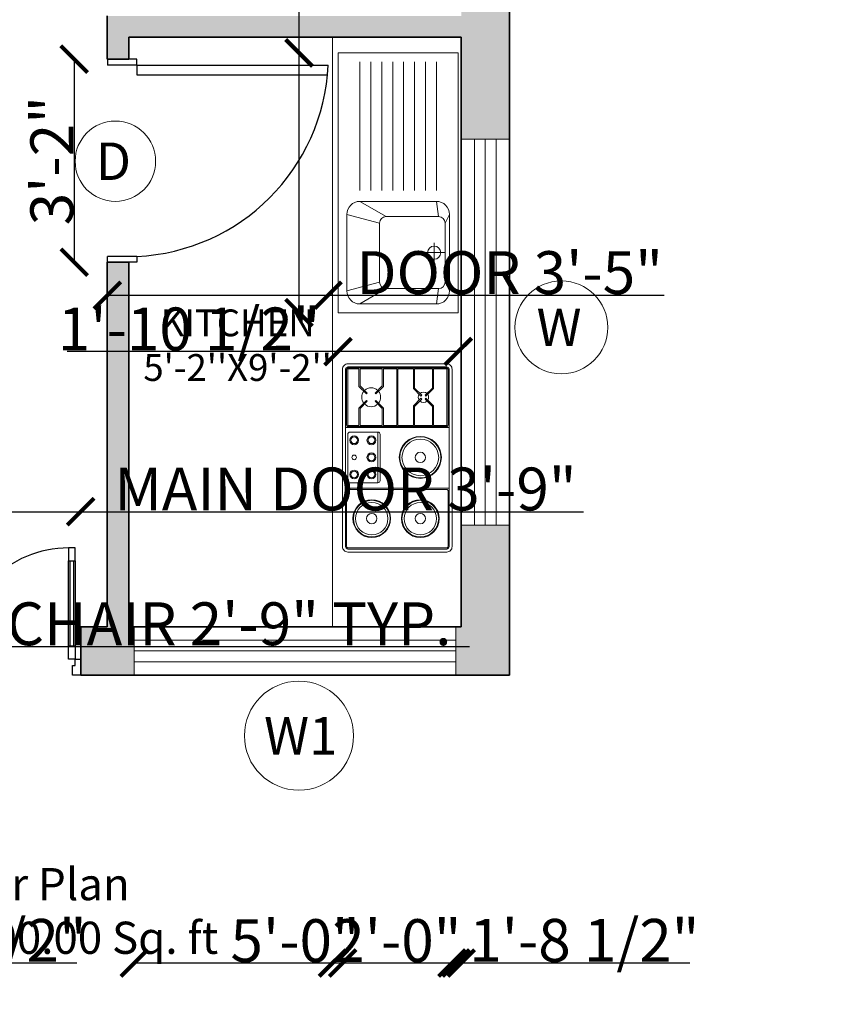
# Model space of a CAD drawing. Units: inches. Extents: x 2209 to 2954, y 1760 to 2265.
# Tile 2 of 7: x 2428 to 2580, y 1761 to 1945. Entities that reach past the tile are written whole.
import ezdxf

# ---------------------------------------------------------------- set-up
doc = ezdxf.new("R2010")
doc.units = ezdxf.units.IN
for name, color, linetype, lineweight in [('A-ANNO-DIMS', 2, 'Continuous', 18), ('A-ANNO-SYMB', 7, 'Continuous', 18), ('A-ANNO-TEXT', 7, 'Continuous', 25), ('A-AREA-IDEN', 7, 'Continuous', 18), ('A-EQPM', 8, 'Continuous', 13), ('A-FLOR-FIXT', 9, 'Continuous', 18), ('A-WALL-PATT', 30, 'Continuous', 13), ('DOOR', 240, 'Continuous', 25), ('KITCHEN', 52, 'Continuous', 20), ('WALL', 7, 'Continuous', 35), ('WINDOW', 190, 'Continuous', 18)]:
    doc.layers.add(name, color=color, linetype=linetype, lineweight=lineweight)
doc.layers.add('A-Glaz', color=92, linetype='Continuous')
doc.layers.add('MAIN DOOR', color=150, linetype='Continuous')
doc.styles.get("Standard").update_dxf_attribs({"font": 'arial.ttf'})
doc.dimstyles.get("Standard").update_dxf_attribs({"dimtxt": 8, "dimasz": 5, "dimexe": 0.18, "dimexo": 0.0625, "dimgap": 0.09, "dimtad": 1, "dimdec": 1, "dimzin": 0, "dimdsep": 46, "dimlunit": 4, "dimtxsty": 'Standard', "dimblk": 'ARCHTICK', "dimcen": 0.09, "dimse1": 1, "dimse2": 1, "dimadec": 0, "dimazin": 0, "dimtfac": 1, "dimtdec": 1, "dimtofl": 0, "dimtmove": 0, "dimatfit": 3, "dimfxl": 1, "dimtolj": 1, "dimtzin": 0, "dimarcsym": 0})

# ---------------------------------------------------------------- blocks, each defined once
blk = doc.blocks.new('A$C13CE0A17')
at = {"layer": 'A-Glaz'}
for p, q in [((0.01, 0.61), (0.01, 0.08)), ((0.03, 0.08), (0.03, 0.61))]:
    blk.add_line(p, q, dxfattribs=at)
blk.add_lwpolyline([(1.4, 0.08), (1.4, 0.61), (1.42, 0.61), (1.42, 0.08)], close=True, dxfattribs=at)
at = {"layer": 'MAIN DOOR'}
for p, q in [((0, 0.61), (0, 0.69)), ((0, 0.69), (0.04, 0.69)), ((0.04, 0.69), (0.04, 0.61)), ((0, 0.61), (0, 0.08)), ((0.04, 0.61), (0, 0.61)), ((0.04, 0.61), (0, 0.61)), ((0.03, 0.61), (0.01, 0.61)), ((0.04, 0.08), (0.04, 0.61)), ((0, 0.08), (0, 0)), ((0.04, 0.08), (0, 0.08)), ((0, 0.08), (0.04, 0.08)), ((0.01, 0.08), (0.03, 0.08)), ((0.04, 0), (0.04, 0.08)), ((-0.035, 0), (-0.035, -0.1)), ((0, 0), (-0.035, 0)), ((0, 0), (0.04, 0)), ((0, -0.04), (0, 0)), ((0.015, -0.04), (0, -0.04)), ((0.015, -0.05), (0.015, -0.04)), ((0.015, -0.1), (0.015, -0.05)), ((-0.035, -0.1), (0.015, -0.1))]:
    blk.add_line(p, q, dxfattribs=at)
for points in [[(1.39, 0.69), (1.39, 0.61), (1.43, 0.61), (1.43, 0.69)], [(1.39, 0.08), (1.39, 0.61), (1.43, 0.61), (1.43, 0.08)], [(1.39, 0), (1.39, 0.08), (1.43, 0.08), (1.43, 0)], [(1.43, 0), (1.465, 0), (1.465, -0.1), (1.415, -0.1), (1.415, -0.05), (1.415, -0.04), (1.43, -0.04)]]:
    blk.add_lwpolyline(points, close=True, dxfattribs=at)
blk.add_arc((1.3872, 0.017), 0.673, 89.76573, 181.44381, dxfattribs=at)
blk.add_ellipse((0.0389, 0.0511), major_axis=(0.6669, -0.1217), ratio=0.940794, start_param=0.11153, end_param=1.73917, dxfattribs=at)
blk = doc.blocks.new('AP0B05')
for p, q in [((35, 100), (35, 880)), ((75, 100), (75, 878.9)), ((35, 100), (11, 100)), ((11, 100), (11, -20)), ((35, 100), (35, -20)), ((815, 100), (815, -20)), ((815, 100), (839, 100)), ((839, 100), (839, -20)), ((11, -20), (35, -20)), ((839, -20), (815, -20))]:
    blk.add_line(p, q)
blk.add_lwpolyline([(35, 100), (75, 100)])
blk.add_arc((-2.4, 62.6), 818.3, 2.6212, 87.3788)
blk = doc.blocks.new('KK')
for p, q in [((0, 0.55), (0, 0)), ((1.19, 0.55), (0, 0.55)), ((1.19, 0), (1.19, 0.55)), ((0.1, 0.51), (0.14, 0.36)), ((0.45, 0.51), (0.1, 0.51)), ((0.41, 0.36), (0.45, 0.51)), ((0.11, 0.33), (0.04, 0.45)), ((0.04, 0.45), (0.04, 0.1)), ((0.44, 0.33), (0.51, 0.45)), ((0.51, 0.1), (0.51, 0.45)), ((0.56, 0.45), (1.15, 0.45)), ((0.56, 0.4), (1.15, 0.4)), ((0.11, 0.09), (0.11, 0.33)), ((0.14, 0.36), (0.41, 0.36)), ((0.44, 0.33), (0.44, 0.09)), ((0.56, 0.35), (1.15, 0.35)), ((0.56, 0.3), (1.15, 0.3)), ((0.56, 0.25), (1.15, 0.25)), ((0.56, 0.2), (1.15, 0.2)), ((0.275, 0.06), (0.275, 0.16)), ((0.56, 0.15), (1.15, 0.15)), ((0.04, 0.1), (0.11, 0.09)), ((0.23, 0.11), (0.32, 0.11)), ((0.44, 0.09), (0.51, 0.1)), ((0.56, 0.1), (1.15, 0.1)), ((0.14, 0.06), (0.1, 0.04)), ((0.41, 0.06), (0.14, 0.06)), ((0.41, 0.06), (0.45, 0.04)), ((0, 0), (1.19, 0)), ((0.1, 0.04), (0.45, 0.04))]:
    blk.add_line(p, q)
blk.add_circle((0.275, 0.11), 0.03)
for centre, radius, start, end in [((0.1, 0.45), 0.06, 90, 180), ((0.45, 0.45), 0.06, 0, 90), ((0.14, 0.33), 0.03, 90, 180), ((0.41, 0.33), 0.03, 0, 90), ((0.1, 0.1), 0.06, 180, 270), ((0.45, 0.1), 0.06, 270, 0), ((0.14, 0.09), 0.03, 180, 270), ((0.41, 0.09), 0.03, 270, 0)]:
    blk.add_arc(centre, radius, start, end)
blk = doc.blocks.new('WIN-W-72IN')
for p, q in [((0, 6.5), (72, 6.5)), ((0, 4.5), (72, 4.5)), ((0, 2.5), (72, 2.5))]:
    blk.add_line(p, q)
blk.add_lwpolyline([(0, 9), (72, 9), (72, 0), (0, 0)], close=True)
blk = doc.blocks.new('TAG-OPENING-W')
blk.add_circle((0, 0), 8.66)
blk.add_text('W', height=7).set_placement((-4.62, -3.5))
blk = doc.blocks.new('TAG-OPENING-D')
blk.add_circle((0, 0), 7.5)
blk.add_text('D', height=7).set_placement((-3.65, -3.5))
blk = doc.blocks.new('_ArchTick')
at = {"color": 0, "linetype": 'ByBlock', "const_width": 0.15}
blk.add_lwpolyline([(-0.5, -0.5), (0.5, 0.5)], dxfattribs=at)
blk = doc.blocks.new('*D47')
at = {"layer": 'A-ANNO-DIMS', "color": 0, "lineweight": -2, "transparency": 16777216}
for p, q in [((2444.15, 1893.15), (2485.33, 1893.15)), ((2485.33, 1893.15), (2548.02, 1893.15))]:
    blk.add_line(p, q, dxfattribs=at)
at = {"layer": 'Defpoints', "color": 0, "transparency": 16777216}
for p in [(2444.15, 1899.32), (2485.33, 1899.32), (2485.33, 1893.15)]:
    blk.add_point(p, dxfattribs=at)
at = {"layer": 'A-ANNO-DIMS', "color": 0, "lineweight": -2, "transparency": 16777216, "xscale": 5, "yscale": 5, "zscale": 5, "rotation": 180}
blk.add_blockref('_ArchTick', (2444.15, 1893.15), dxfattribs=at)
at = {"layer": 'A-ANNO-DIMS', "color": 0, "lineweight": -2, "transparency": 16777216, "xscale": 5, "yscale": 5, "zscale": 5}
blk.add_blockref('_ArchTick', (2485.33, 1893.15), dxfattribs=at)
at = {"layer": 'A-ANNO-DIMS', "color": 0, "transparency": 16777216, "insert": (2519.18, 1897.38), "char_height": 8, "attachment_point": 5}
blk.add_mtext('\\A1;DOOR 3\'-5"', dxfattribs=at)
blk = doc.blocks.new('*D48')
at = {"layer": 'A-ANNO-DIMS', "color": 0, "lineweight": -2, "transparency": 16777216}
blk.add_line((2437.98, 1937.21), (2437.98, 1899.32), dxfattribs=at)
at = {"layer": 'Defpoints', "color": 0, "transparency": 16777216}
for p in [(2444.15, 1937.21), (2437.98, 1899.32), (2444.15, 1899.32)]:
    blk.add_point(p, dxfattribs=at)
at = {"layer": 'A-ANNO-DIMS', "color": 0, "lineweight": -2, "transparency": 16777216, "xscale": 5, "yscale": 5, "zscale": 5}
for p, rotation in [((2437.98, 1937.21), 90), ((2437.98, 1899.32), 270)]:
    blk.add_blockref('_ArchTick', p, dxfattribs=dict(at, rotation=rotation))
at = {"layer": 'A-ANNO-DIMS', "color": 0, "transparency": 16777216, "insert": (2433.8, 1918.27), "char_height": 8, "attachment_point": 5, "rotation": 90}
blk.add_mtext('\\A1;3\'-2"', dxfattribs=at)
blk = doc.blocks.new('*D49')
at = {"layer": 'A-ANNO-DIMS', "color": 0, "lineweight": -2, "transparency": 16777216}
for p, q in [((2394.15, 1852.78), (2439.18, 1852.78)), ((2439.18, 1852.78), (2532.94, 1852.78))]:
    blk.add_line(p, q, dxfattribs=at)
at = {"layer": 'Defpoints', "color": 0, "transparency": 16777216}
for p in [(2439.18, 1852.78), (2394.15, 1846.02), (2439.18, 1846.02)]:
    blk.add_point(p, dxfattribs=at)
at = {"layer": 'A-ANNO-DIMS', "color": 0, "lineweight": -2, "transparency": 16777216, "xscale": 5, "yscale": 5, "zscale": 5, "rotation": 180}
blk.add_blockref('_ArchTick', (2394.15, 1852.78), dxfattribs=at)
at = {"layer": 'A-ANNO-DIMS', "color": 0, "lineweight": -2, "transparency": 16777216, "xscale": 5, "yscale": 5, "zscale": 5}
blk.add_blockref('_ArchTick', (2439.18, 1852.78), dxfattribs=at)
at = {"layer": 'A-ANNO-DIMS', "color": 0, "transparency": 16777216, "insert": (2488.56, 1857.01), "char_height": 8, "attachment_point": 5}
blk.add_mtext('\\A1;MAIN DOOR 3\'-9"', dxfattribs=at)
blk = doc.blocks.new('*D59')
at = {"layer": 'A-ANNO-DIMS', "color": 0, "lineweight": -2, "transparency": 16777216}
for p, q in [((2361.69, 1827.63), (2394.59, 1827.63)), ((2394.59, 1827.63), (2511.71, 1827.63))]:
    blk.add_line(p, q, dxfattribs=at)
at = {"layer": 'Defpoints', "color": 0, "transparency": 16777216}
for p in [(2361.69, 1832.57), (2394.59, 1832.57), (2394.59, 1827.63)]:
    blk.add_point(p, dxfattribs=at)
at = {"layer": 'A-ANNO-DIMS', "color": 0, "lineweight": -2, "transparency": 16777216, "xscale": 5, "yscale": 5, "zscale": 5, "rotation": 180}
blk.add_blockref('_ArchTick', (2361.69, 1827.63), dxfattribs=at)
at = {"layer": 'A-ANNO-DIMS', "color": 0, "lineweight": -2, "transparency": 16777216, "xscale": 5, "yscale": 5, "zscale": 5}
blk.add_blockref('_ArchTick', (2394.59, 1827.63), dxfattribs=at)
at = {"layer": 'A-ANNO-DIMS', "color": 0, "transparency": 16777216, "insert": (2455.65, 1831.86), "char_height": 8, "attachment_point": 5}
blk.add_mtext('\\A1;ARMCHAIR 2\'-9" TYP.', dxfattribs=at)
blk = doc.blocks.new('*D65')
at = {"layer": 'A-ANNO-DIMS', "color": 0, "lineweight": -2, "transparency": 16777216}
for p, q in [((2479.92, 1938.37), (2479.92, 2121.89)), ((2479.92, 1889.91), (2479.92, 1938.37))]:
    blk.add_line(p, q, dxfattribs=at)
at = {"layer": 'Defpoints', "color": 0, "transparency": 16777216}
for p in [(2479.92, 1938.37), (2487.19, 1938.37), (2487.19, 1889.91)]:
    blk.add_point(p, dxfattribs=at)
at = {"layer": 'A-ANNO-DIMS', "color": 0, "lineweight": -2, "transparency": 16777216, "xscale": 5, "yscale": 5, "zscale": 5}
for p, rotation in [((2479.92, 1938.37), 90), ((2479.92, 1889.91), 270)]:
    blk.add_blockref('_ArchTick', p, dxfattribs=dict(at, rotation=rotation))
at = {"layer": 'A-ANNO-DIMS', "color": 0, "transparency": 16777216, "insert": (2475.69, 2032.63), "char_height": 8, "attachment_point": 5, "rotation": 90}
blk.add_mtext('\\A1;SINK WITH DRAINBOARD 4\'-0 1/2"', dxfattribs=at)
blk = doc.blocks.new('*D66')
at = {"layer": 'A-ANNO-DIMS', "color": 0, "lineweight": -2, "transparency": 16777216}
for p, q in [((2487.19, 1882.64), (2436.64, 1882.64)), ((2509.59, 1882.64), (2487.19, 1882.64))]:
    blk.add_line(p, q, dxfattribs=at)
at = {"layer": 'Defpoints', "color": 0, "transparency": 16777216}
for p in [(2487.19, 1889.91), (2509.59, 1889.91), (2487.19, 1882.64)]:
    blk.add_point(p, dxfattribs=at)
at = {"layer": 'A-ANNO-DIMS', "color": 0, "lineweight": -2, "transparency": 16777216, "xscale": 5, "yscale": 5, "zscale": 5, "rotation": 180}
blk.add_blockref('_ArchTick', (2487.19, 1882.64), dxfattribs=at)
at = {"layer": 'A-ANNO-DIMS', "color": 0, "lineweight": -2, "transparency": 16777216, "xscale": 5, "yscale": 5, "zscale": 5}
blk.add_blockref('_ArchTick', (2509.59, 1882.64), dxfattribs=at)
at = {"layer": 'A-ANNO-DIMS', "color": 0, "transparency": 16777216, "insert": (2459.42, 1886.87), "char_height": 8, "attachment_point": 5}
blk.add_mtext('\\A1;1\'-10 1/2"', dxfattribs=at)
blk = doc.blocks.new('*D67')
at = {"layer": 'A-ANNO-DIMS', "color": 0, "lineweight": -2, "transparency": 16777216}
blk.add_line((2449.17, 1768.57), (2509.17, 1768.57), dxfattribs=at)
at = {"layer": 'Defpoints', "color": 0, "transparency": 16777216}
for p in [(2449.17, 1822.29), (2509.17, 1822.29), (2509.17, 1768.57)]:
    blk.add_point(p, dxfattribs=at)
at = {"layer": 'A-ANNO-DIMS', "color": 0, "lineweight": -2, "transparency": 16777216, "xscale": 5, "yscale": 5, "zscale": 5, "rotation": 180}
blk.add_blockref('_ArchTick', (2449.17, 1768.57), dxfattribs=at)
at = {"layer": 'A-ANNO-DIMS', "color": 0, "lineweight": -2, "transparency": 16777216, "xscale": 5, "yscale": 5, "zscale": 5}
blk.add_blockref('_ArchTick', (2509.17, 1768.57), dxfattribs=at)
at = {"layer": 'A-ANNO-DIMS', "color": 0, "transparency": 16777216, "insert": (2479.17, 1772.74), "char_height": 8, "attachment_point": 5}
blk.add_mtext('\\A1;5\'-0"', dxfattribs=at)
blk = doc.blocks.new('*D69')
at = {"layer": 'A-ANNO-DIMS', "color": 0, "lineweight": -2, "transparency": 16777216}
for p, q in [((2372.65, 1768.57), (2394.15, 1768.57)), ((2394.15, 1768.57), (2438.49, 1768.57))]:
    blk.add_line(p, q, dxfattribs=at)
at = {"layer": 'Defpoints', "color": 0, "transparency": 16777216}
for p in [(2372.65, 1822.29), (2394.15, 1822.29), (2394.15, 1768.57)]:
    blk.add_point(p, dxfattribs=at)
at = {"layer": 'A-ANNO-DIMS', "color": 0, "lineweight": -2, "transparency": 16777216, "xscale": 5, "yscale": 5, "zscale": 5, "rotation": 180}
blk.add_blockref('_ArchTick', (2372.65, 1768.57), dxfattribs=at)
at = {"layer": 'A-ANNO-DIMS', "color": 0, "lineweight": -2, "transparency": 16777216, "xscale": 5, "yscale": 5, "zscale": 5}
blk.add_blockref('_ArchTick', (2394.15, 1768.57), dxfattribs=at)
at = {"layer": 'A-ANNO-DIMS', "color": 0, "transparency": 16777216, "insert": (2418.82, 1772.79), "char_height": 8, "attachment_point": 5}
blk.add_mtext('\\A1;1\'-9 1/2"', dxfattribs=at)
blk = doc.blocks.new('*D74')
at = {"layer": 'A-ANNO-DIMS', "color": 0, "lineweight": -2, "transparency": 16777216}
blk.add_line((2920.04, 1822.29), (2920.04, 1850.29), dxfattribs=at)
at = {"layer": 'Defpoints', "color": 0, "transparency": 16777216}
for p in [(2519.15, 1850.29), (2920.04, 1850.29), (2519.15, 1822.29)]:
    blk.add_point(p, dxfattribs=at)
at = {"layer": 'A-ANNO-DIMS', "color": 0, "lineweight": -2, "transparency": 16777216, "xscale": 5, "yscale": 5, "zscale": 5}
for p, rotation in [((2920.04, 1850.29), 90), ((2920.04, 1822.29), 270)]:
    blk.add_blockref('_ArchTick', p, dxfattribs=dict(at, rotation=rotation))
at = {"layer": 'A-ANNO-DIMS', "color": 0, "transparency": 16777216, "insert": (2915.94, 1836.29), "char_height": 8, "attachment_point": 5, "rotation": 90}
blk.add_mtext('\\A1;2\'-4"', dxfattribs=at)
blk = doc.blocks.new('*D75')
at = {"layer": 'A-ANNO-DIMS', "color": 0, "lineweight": -2, "transparency": 16777216}
blk.add_line((2920.04, 1922.29), (2920.04, 1971.25), dxfattribs=at)
at = {"layer": 'Defpoints', "color": 0, "transparency": 16777216}
for p in [(2519.15, 1971.25), (2920.04, 1971.25), (2519.15, 1922.29)]:
    blk.add_point(p, dxfattribs=at)
at = {"layer": 'A-ANNO-DIMS', "color": 0, "lineweight": -2, "transparency": 16777216, "xscale": 5, "yscale": 5, "zscale": 5}
for p, rotation in [((2920.04, 1971.25), 90), ((2920.04, 1922.29), 270)]:
    blk.add_blockref('_ArchTick', p, dxfattribs=dict(at, rotation=rotation))
at = {"layer": 'A-ANNO-DIMS', "color": 0, "transparency": 16777216, "insert": (2915.94, 1946.77), "char_height": 8, "attachment_point": 5, "rotation": 90}
blk.add_mtext('\\A1;4\'-1"', dxfattribs=at)
blk = doc.blocks.new('*D80')
at = {"layer": 'A-ANNO-DIMS', "color": 0, "lineweight": -2, "transparency": 16777216}
blk.add_line((2920.04, 1831.29), (2920.04, 1889.91), dxfattribs=at)
at = {"layer": 'Defpoints', "color": 0, "transparency": 16777216}
for p in [(2509.59, 1889.91), (2920.04, 1889.91), (2510.15, 1831.29)]:
    blk.add_point(p, dxfattribs=at)
at = {"layer": 'A-ANNO-DIMS', "color": 0, "lineweight": -2, "transparency": 16777216, "xscale": 5, "yscale": 5, "zscale": 5}
for p, rotation in [((2920.04, 1889.91), 90), ((2920.04, 1831.29), 270)]:
    blk.add_blockref('_ArchTick', p, dxfattribs=dict(at, rotation=rotation))
at = {"layer": 'A-ANNO-DIMS', "color": 0, "transparency": 16777216, "insert": (2915.82, 1860.6), "char_height": 8, "attachment_point": 5, "rotation": 90}
blk.add_mtext('\\A1;4\'-10 1/2"', dxfattribs=at)
blk = doc.blocks.new('*D81')
at = {"layer": 'A-ANNO-DIMS', "color": 0, "lineweight": -2, "transparency": 16777216}
blk.add_line((2486.15, 1768.57), (2510.15, 1768.57), dxfattribs=at)
at = {"layer": 'Defpoints', "color": 0, "transparency": 16777216}
for p in [(2486.15, 1831.29), (2510.15, 1831.29), (2510.15, 1768.57)]:
    blk.add_point(p, dxfattribs=at)
at = {"layer": 'A-ANNO-DIMS', "color": 0, "lineweight": -2, "transparency": 16777216, "xscale": 5, "yscale": 5, "zscale": 5, "rotation": 180}
blk.add_blockref('_ArchTick', (2486.15, 1768.57), dxfattribs=at)
at = {"layer": 'A-ANNO-DIMS', "color": 0, "lineweight": -2, "transparency": 16777216, "xscale": 5, "yscale": 5, "zscale": 5}
blk.add_blockref('_ArchTick', (2510.15, 1768.57), dxfattribs=at)
at = {"layer": 'A-ANNO-DIMS', "color": 0, "transparency": 16777216, "insert": (2498.15, 1772.74), "char_height": 8, "attachment_point": 5}
blk.add_mtext('\\A1;2\'-0"', dxfattribs=at)
blk = doc.blocks.new('*D82')
at = {"layer": 'A-ANNO-DIMS', "color": 0, "lineweight": -2, "transparency": 16777216}
for p, q in [((2488.02, 1768.57), (2508.45, 1768.57)), ((2508.45, 1768.57), (2552.79, 1768.57))]:
    blk.add_line(p, q, dxfattribs=at)
at = {"layer": 'Defpoints', "color": 0, "transparency": 16777216}
for p in [(2488.02, 1846.26), (2508.45, 1846.26), (2508.45, 1768.57)]:
    blk.add_point(p, dxfattribs=at)
at = {"layer": 'A-ANNO-DIMS', "color": 0, "lineweight": -2, "transparency": 16777216, "xscale": 5, "yscale": 5, "zscale": 5, "rotation": 180}
blk.add_blockref('_ArchTick', (2488.02, 1768.57), dxfattribs=at)
at = {"layer": 'A-ANNO-DIMS', "color": 0, "lineweight": -2, "transparency": 16777216, "xscale": 5, "yscale": 5, "zscale": 5}
blk.add_blockref('_ArchTick', (2508.45, 1768.57), dxfattribs=at)
at = {"layer": 'A-ANNO-DIMS', "color": 0, "transparency": 16777216, "insert": (2533.12, 1772.79), "char_height": 8, "attachment_point": 5}
blk.add_mtext('\\A1;1\'-8 1/2"', dxfattribs=at)
blk = doc.blocks.new('*D83')
at = {"layer": 'A-ANNO-DIMS', "color": 0, "lineweight": -2, "transparency": 16777216}
blk.add_line((2224.78, 1845.25), (2224.78, 1880.36), dxfattribs=at)
at = {"layer": 'Defpoints', "color": 0, "transparency": 16777216}
for p in [(2224.78, 1880.36), (2489.03, 1880.36), (2489.03, 1845.25)]:
    blk.add_point(p, dxfattribs=at)
at = {"layer": 'A-ANNO-DIMS', "color": 0, "lineweight": -2, "transparency": 16777216, "xscale": 5, "yscale": 5, "zscale": 5}
for p, rotation in [((2224.78, 1880.36), 90), ((2224.78, 1845.25), 270)]:
    blk.add_blockref('_ArchTick', p, dxfattribs=dict(at, rotation=rotation))
at = {"layer": 'A-ANNO-DIMS', "color": 0, "transparency": 16777216, "insert": (2220.67, 1862.81), "char_height": 8, "attachment_point": 5, "rotation": 90}
blk.add_mtext('\\A1;2\'-11"', dxfattribs=at)
blk = doc.blocks.new('*D84')
at = {"layer": 'A-ANNO-DIMS', "color": 0, "lineweight": -2, "transparency": 16777216}
for p, q in [((2224.78, 1845.25), (2224.78, 1870.94)), ((2224.78, 1831.29), (2224.78, 1845.25))]:
    blk.add_line(p, q, dxfattribs=at)
at = {"layer": 'Defpoints', "color": 0, "transparency": 16777216}
for p in [(2224.78, 1845.25), (2489.03, 1845.25), (2486.15, 1831.29)]:
    blk.add_point(p, dxfattribs=at)
at = {"layer": 'A-ANNO-DIMS', "color": 0, "lineweight": -2, "transparency": 16777216, "xscale": 5, "yscale": 5, "zscale": 5}
for p, rotation in [((2224.78, 1845.25), 90), ((2224.78, 1831.29), 270)]:
    blk.add_blockref('_ArchTick', p, dxfattribs=dict(at, rotation=rotation))
at = {"layer": 'A-ANNO-DIMS', "color": 0, "transparency": 16777216, "insert": (2220.67, 1860.6), "char_height": 8, "attachment_point": 5, "rotation": 90}
blk.add_mtext('\\A1;1\'-2"', dxfattribs=at)
blk = doc.blocks.new('*D88')
at = {"layer": 'A-ANNO-DIMS', "color": 0, "lineweight": -2, "transparency": 16777216}
blk.add_line((2224.78, 1919.53), (2224.78, 1973.14), dxfattribs=at)
at = {"layer": 'Defpoints', "color": 0, "transparency": 16777216}
for p in [(2224.78, 1973.14), (2629.22, 1973.14), (2629.22, 1919.53)]:
    blk.add_point(p, dxfattribs=at)
at = {"layer": 'A-ANNO-DIMS', "color": 0, "lineweight": -2, "transparency": 16777216, "xscale": 5, "yscale": 5, "zscale": 5}
for p, rotation in [((2224.78, 1973.14), 90), ((2224.78, 1919.53), 270)]:
    blk.add_blockref('_ArchTick', p, dxfattribs=dict(at, rotation=rotation))
at = {"layer": 'A-ANNO-DIMS', "color": 0, "transparency": 16777216, "insert": (2220.55, 1946.34), "char_height": 8, "attachment_point": 5, "rotation": 90}
blk.add_mtext('\\A1;4\'-5 1/2"', dxfattribs=at)

msp = doc.modelspace()

# ---------------------------------------------------------------- hatches: boundary and pattern name
at = {"layer": 'A-WALL-PATT', "transparency": 33554585}
h = msp.add_hatch(color=256, dxfattribs=at)
h.dxf.hatch_style = 1
h.paths.add_polyline_path([(2519.15, 2182.29), (2402.15, 2182.29), (2402.15, 2173.29), (2444.15, 2173.29), (2444.15, 2154.12), (2448.15, 2154.12), (2448.15, 2173.29), (2510.15, 2173.29), (2510.15, 2167.29), (2519.15, 2167.29)])
h.paths.add_polyline_path([(2330.15, 2182.29), (2279.15, 2182.29), (2279.15, 2145.83), (2288.15, 2145.83), (2288.15, 2158.01), (2288.15, 2173.29), (2330.15, 2173.29)])
h.paths.add_polyline_path([(2288.15, 2073.83), (2279.15, 2073.83), (2279.15, 2009.29), (2288.15, 2009.29), (2288.15, 2037.29), (2404.15, 2037.29), (2404.15, 2041.29), (2288.15, 2041.29)])
h.paths.add_polyline_path([(2519.15, 2131.29), (2510.15, 2131.29), (2510.15, 2125.29), (2444.15, 2125.29), (2444.15, 2041.29), (2439.11, 2041.29), (2439.11, 2037.29), (2448.15, 2037.29), (2448.15, 2069.29), (2481.65, 2069.29), (2481.65, 2073.29), (2448.15, 2073.29), (2448.15, 2121.29), (2468.19, 2121.29), (2468.19, 2121.32), (2488.37, 2121.32), (2510.15, 2121.29), (2510.15, 2113.63), (2519.15, 2113.63)])
h.paths.add_polyline_path([(2519.15, 2077.63), (2510.15, 2077.63), (2510.15, 2073.32), (2510.17, 2073.32), (2510.15, 2069.19), (2510.15, 2043.25), (2519.15, 2043.25)], flags=17)
h.paths.add_polyline_path([(2519.15, 1971.25), (2510.15, 1971.25), (2510.15, 1945.29), (2444.15, 1945.29), (2444.15, 1937.21), (2448.15, 1937.21), (2448.15, 1941.29), (2510.15, 1941.29), (2510.15, 1922.29), (2519.15, 1922.29)])
h.paths.add_polyline_path([(2288.15, 1941.29), (2394.15, 1941.29), (2394.15, 1945.29), (2288.15, 1945.29), (2288.15, 1973.29), (2279.15, 1973.29), (2279.15, 1919.97), (2288.15, 1919.97)])
h.paths.add_polyline_path([(2300.65, 1831.29), (2288.15, 1831.29), (2288.15, 1847.97), (2279.15, 1847.97), (2279.15, 1822.29), (2300.65, 1822.29)])
h.paths.add_polyline_path([(2394.15, 1825.29), (2394.15, 1831.29), (2372.65, 1831.29), (2372.65, 1822.29), (2394.15, 1822.29)])
h.paths.add_polyline_path([(2449.17, 1831.29), (2448.15, 1831.29), (2448.15, 1899.32), (2444.15, 1899.32), (2444.15, 1831.29), (2439.18, 1831.29), (2439.18, 1822.29), (2449.17, 1822.29)])
h.paths.add_polyline_path([(2519.15, 1850.29), (2510.15, 1850.29), (2510.15, 1831.29), (2509.17, 1831.29), (2509.17, 1822.29), (2519.15, 1822.29)])
h.paths.add_polyline_path([(2638.22, 1941.29), (2744.22, 1941.29), (2744.22, 1945.29), (2638.22, 1945.29), (2638.22, 1973.14), (2629.22, 1973.14), (2629.22, 1919.53), (2638.22, 1919.53)])
h.paths.add_polyline_path([(2638.22, 1847.53), (2629.22, 1847.53), (2629.22, 1822.29), (2650.72, 1822.29), (2650.72, 1831.29), (2638.22, 1831.29)])
h.paths.add_polyline_path([(2638.22, 2037.29), (2754.22, 2037.29), (2754.22, 2041.29), (2638.22, 2041.29), (2638.22, 2074.27), (2629.22, 2074.27), (2629.22, 2009.14), (2638.22, 2009.14)])
h.paths.add_polyline_path([(2803.22, 1936.29), (2812.78, 1936.29), (2812.78, 1945.29), (2791.22, 1945.29), (2791.22, 1936.29), (2794.22, 1936.29), (2794.22, 1831.29), (2722.72, 1831.29), (2722.72, 1822.29), (2803.22, 1822.29)])
h.paths.add_polyline_path([(2869.22, 1955.43), (2860.22, 1955.43), (2860.22, 1945.29), (2853.36, 1945.29), (2853.36, 1936.29), (2869.22, 1936.29)])
h.paths.add_polyline_path([(2680.22, 2182.29), (2629.22, 2182.29), (2629.22, 2146.27), (2638.22, 2146.27), (2638.22, 2173.29), (2680.22, 2173.29)])
h.paths.add_polyline_path([(2869.22, 2182.29), (2752.22, 2182.29), (2752.22, 2173.29), (2794.22, 2173.29), (2794.22, 2142.92), (2798.22, 2142.92), (2798.22, 2173.29), (2860.22, 2173.29), (2860.22, 2158.46), (2869.22, 2158.46)])
h.paths.add_polyline_path([(2869.22, 2122.46), (2860.22, 2122.46), (2860.22, 2090.29), (2869.22, 2090.29)])

# ---------------------------------------------------------------- linework, layer by layer
at = {"layer": 'A-ANNO-SYMB'}
msp.add_circle((2479.89, 1810.98), 10.17, dxfattribs=at)
at = {"layer": 'A-EQPM'}
for p, q in [((2498.14, 1868.87), (2498.14, 1879.4)), ((2498.34, 1868.87), (2498.34, 1879.4)), ((2488.58, 1868.47), (2507.89, 1868.47)), ((2488.99, 1867.23), (2488.99, 1858.58)), ((2494.62, 1867.63), (2489.39, 1867.63)), ((2494.62, 1867.63), (2494.62, 1858.18)), ((2495.02, 1867.23), (2495.02, 1858.58)), ((2489.39, 1858.18), (2494.62, 1858.18)), ((2488.58, 1857.14), (2507.89, 1857.14))]:
    msp.add_line(p, q, dxfattribs=at)
for points in [[(2508.45, 1879.36), (2508.45, 1846.26, -0.414214), (2507.45, 1845.25), (2489.03, 1845.25, -0.414214), (2488.02, 1846.26), (2488.02, 1879.36, -0.414214), (2489.03, 1880.36), (2507.45, 1880.36, -0.414214)], [(2507.89, 1879.36), (2507.89, 1846.26, -0.414214), (2507.45, 1845.81), (2489.03, 1845.81, -0.414214), (2488.58, 1846.26), (2488.58, 1879.36, -0.414214), (2489.03, 1879.8), (2507.45, 1879.8, -0.414214)], [(2507.69, 1868.91), (2507.69, 1879.36, 0.414214), (2507.45, 1879.6), (2489.03, 1879.6, 0.414214), (2488.78, 1879.36), (2488.78, 1868.91, 0.414214), (2489.03, 1868.67), (2507.45, 1868.67, 0.414214)], [(2507.69, 1856.7), (2507.69, 1846.26, -0.414214), (2507.45, 1846.01), (2489.03, 1846.01, -0.414214), (2488.78, 1846.26), (2488.78, 1856.7, -0.414214), (2489.03, 1856.94), (2507.45, 1856.94, -0.414214)]]:
    msp.add_lwpolyline(points, format="xyb", close=True, dxfattribs=at)
for points in [[(2491.09, 1879.4), (2489.03, 1879.4, 0.414214), (2488.99, 1879.36), (2488.99, 1868.91, 0.414214), (2489.03, 1868.87), (2491.09, 1868.87)], [(2504.98, 1868.87), (2507.45, 1868.87, 0.414214), (2507.49, 1868.91), (2507.49, 1879.36, 0.414214), (2507.45, 1879.4), (2504.98, 1879.4)]]:
    msp.add_lwpolyline(points, format="xyb", dxfattribs=at)
for points in [[(2491.09, 1879.4), (2491.09, 1876.16), (2492.49, 1874.75), (2492.64, 1874.89), (2491.29, 1876.24), (2491.29, 1879.4)], [(2495.43, 1879.4), (2491.29, 1879.4)], [(2495.63, 1879.4), (2495.63, 1876.16), (2494.22, 1874.75), (2494.08, 1874.89), (2495.43, 1876.24), (2495.43, 1879.4)], [(2498.14, 1879.4), (2495.63, 1879.4)], [(2501.24, 1879.4), (2498.34, 1879.4)], [(2501.24, 1879.4), (2501.24, 1875.76), (2502.65, 1874.35), (2502.79, 1874.49), (2501.44, 1875.84), (2501.44, 1879.4)], [(2504.78, 1879.4), (2501.44, 1879.4)], [(2504.98, 1879.4), (2504.98, 1875.76), (2503.58, 1874.35), (2503.43, 1874.49), (2504.78, 1875.84), (2504.78, 1879.4)], [(2501.44, 1868.87), (2501.44, 1872.43), (2502.79, 1873.78), (2502.65, 1873.93), (2501.24, 1872.52), (2501.24, 1868.87)], [(2504.78, 1868.87), (2504.78, 1872.43), (2503.43, 1873.78), (2503.58, 1873.93), (2504.98, 1872.52), (2504.98, 1868.87)], [(2491.29, 1868.87), (2491.29, 1872.03), (2492.64, 1873.38), (2492.49, 1873.52), (2491.09, 1872.12), (2491.09, 1868.87)], [(2495.43, 1868.87), (2495.43, 1872.03), (2494.08, 1873.38), (2494.22, 1873.52), (2495.63, 1872.12), (2495.63, 1868.87)], [(2491.29, 1868.87), (2495.43, 1868.87)], [(2495.63, 1868.87), (2498.14, 1868.87)], [(2498.34, 1868.87), (2501.24, 1868.87)], [(2501.44, 1868.87), (2504.78, 1868.87)]]:
    msp.add_lwpolyline(points, dxfattribs=at)
for centre, radius in [((2490.19, 1866.1), 0.83), ((2490.19, 1866.1), 0.629), ((2493.41, 1866.1), 0.83), ((2493.41, 1866.1), 0.629), ((2502.53, 1862.91), 3.92), ((2502.53, 1862.91), 3.82), ((2502.53, 1862.91), 3.42), ((2490.19, 1862.91), 0.428), ((2493.41, 1862.91), 0.83), ((2493.41, 1862.91), 0.629), ((2502.53, 1862.91), 0.965), ((2490.19, 1859.72), 0.83), ((2490.19, 1859.72), 0.629), ((2493.41, 1859.72), 0.83), ((2493.41, 1859.72), 0.629), ((2493.47, 1851.48), 3.52), ((2493.47, 1851.48), 3.42), ((2493.47, 1851.48), 3.02), ((2502.53, 1851.48), 3.52), ((2502.53, 1851.48), 3.42), ((2502.53, 1851.48), 3.02), ((2493.47, 1851.48), 0.965), ((2502.53, 1851.48), 0.965)]:
    msp.add_circle(centre, radius, dxfattribs=at)
for centre, radius, start, end in [((2493.36, 1874.14), 1.77, 45.756, 134.244), ((2493.36, 1874.14), 1.77, 140.7646, 219.2354), ((2493.36, 1874.14), 1.77, 320.7646, 39.2354), ((2503.11, 1874.14), 0.965, 145.6111, 214.3889), ((2503.11, 1874.14), 0.965, 46.3862, 133.6138), ((2503.11, 1874.14), 0.965, 325.6111, 34.3889), ((2493.36, 1874.14), 1.77, 225.756, 314.244), ((2503.11, 1874.14), 0.965, 226.3862, 313.6138), ((2489.39, 1867.23), 0.402, 90, 180), ((2494.62, 1867.23), 0.402, 0, 90), ((2489.39, 1858.58), 0.402, 180, 270), ((2494.62, 1858.58), 0.402, 270, 0)]:
    msp.add_arc(centre, radius, start, end, dxfattribs=at)
at = {"layer": 'KITCHEN'}
msp.add_line((2486.15, 1941.29), (2486.15, 1831.29), dxfattribs=at)
at = {"layer": 'WALL'}
for p, q in [((2519.15, 2182.29), (2519.15, 1822.29)), ((2444.15, 1945.29), (2444.15, 1937.21)), ((2448.15, 1941.29), (2448.15, 1937.21)), ((2448.15, 1941.29), (2510.15, 1941.29)), ((2510.15, 1941.29), (2510.15, 1831.29)), ((2444.15, 1937.21), (2448.15, 1937.21)), ((2444.15, 1899.32), (2448.15, 1899.32)), ((2444.15, 1899.32), (2444.15, 1831.29)), ((2448.15, 1899.32), (2448.15, 1831.29)), ((2439.18, 1831.29), (2439.18, 1822.29)), ((2439.18, 1831.29), (2444.15, 1831.29)), ((2448.15, 1831.29), (2510.15, 1831.29)), ((2439.18, 1822.29), (2519.15, 1822.29))]:
    msp.add_line(p, q, dxfattribs=at)
at = {"layer": 'WINDOW'}
for p, q in [((2449.17, 1828.79), (2509.17, 1828.79)), ((2449.17, 1826.79), (2509.17, 1826.79)), ((2449.17, 1824.79), (2509.17, 1824.79))]:
    msp.add_line(p, q, dxfattribs=at)
msp.add_lwpolyline([(2449.17, 1831.29), (2509.17, 1831.29), (2509.17, 1822.29), (2449.17, 1822.29)], close=True, dxfattribs=at)

# ---------------------------------------------------------------- block references
at = {"layer": 'A-ANNO-SYMB'}
for name, p in [('TAG-OPENING-D', (2445.65, 1918.16)), ('TAG-OPENING-W', (2528.83, 1887.16))]:
    msp.add_blockref(name, p, dxfattribs=at)
at = {"layer": 'A-FLOR-FIXT', "xscale": 40.72201486386835, "yscale": 40.72201486386835, "zscale": 40.72201486386835, "rotation": 90}
msp.add_blockref('KK', (2509.59, 1889.91), dxfattribs=at)
at = {"layer": 'DOOR', "xscale": 0.0457560220064254, "yscale": 0.0457560220064254, "zscale": 0.0457560220064254, "rotation": 270}
msp.add_blockref('AP0B05', (2445.07, 1937.71), dxfattribs=at)
at = {"layer": 'DOOR', "xscale": 30.0188950098318, "yscale": 30.0188950098318, "zscale": 30.0188950098318}
msp.add_blockref('A$C13CE0A17', (2395.21, 1825.29), dxfattribs=at)
at = {"layer": 'WINDOW', "rotation": 90.00000000000033}
msp.add_blockref('WIN-W-72IN', (2519.15, 1850.28), dxfattribs=at)

# ---------------------------------------------------------------- texts
at = {"layer": 'A-ANNO-SYMB'}
msp.add_text('W1', height=7, dxfattribs=at).set_placement((2473.39, 1807.46))
at = {"layer": 'A-ANNO-TEXT', "insert": (2338.03, 1786.28), "char_height": 6, "attachment_point": 1}
msp.add_mtext_dynamic_manual_height_columns('\\pxqc;Ground Floor Plan\\PBuilt Up Area : 600.00 Sq. ft', width=151.0778, gutter_width=102.73, heights=[0], dxfattribs=at)
at = {"layer": 'A-AREA-IDEN', "insert": (2445.88, 1890.51), "char_height": 5, "attachment_point": 1}
msp.add_mtext_dynamic_manual_height_columns("\\pxqc;KITCHEN\\P5'-2''X9'-2''", width=45.1409, gutter_width=12.5, heights=[0], dxfattribs=at)

# ---------------------------------------------------------------- dimensions: what is measured, and where the dimension line sits
at = {"layer": 'A-ANNO-DIMS'}
dim = msp.add_linear_dim(base=(2479.92, 1938.37), p1=(2487.19, 1889.91), p2=(2487.19, 1938.37), angle=90, text='SINK WITH DRAINBOARD <>', dimstyle='Standard', override={"dimdec": 1, "dimlfac": 1, "dimrnd": 0, "dimzin": 1, "dimdsep": 46, "dimlunit": 4, "dimfrac": 2}, dxfattribs=at)
dim.commit()
dim.dimension.update_dxf_attribs({"geometry": '*D65', "text_midpoint": (2475.69, 2032.63)})
for base, p1, p2, angle, picture, middle in [((2224.78, 1973.14), (2629.22, 1919.53), (2629.22, 1973.14), 90, '*D88', (2220.55, 1946.34)), ((2920.04, 1971.25), (2519.15, 1922.29), (2519.15, 1971.25), 90, '*D75', (2915.94, 1946.77)), ((2437.98, 1899.32), (2444.15, 1937.21), (2444.15, 1899.32), 270, '*D48', (2433.8, 1918.27)), ((2487.19, 1882.64), (2509.59, 1889.91), (2487.19, 1889.91), 180, '*D66', (2459.42, 1886.87)), ((2920.04, 1889.91), (2510.15, 1831.29), (2509.59, 1889.91), 90, '*D80', (2915.82, 1860.6)), ((2224.78, 1880.36), (2489.03, 1845.25), (2489.03, 1880.36), 90, '*D83', (2220.67, 1862.81)), ((2224.78, 1845.25), (2486.15, 1831.29), (2489.03, 1845.25), 90, '*D84', (2220.67, 1860.6)), ((2920.04, 1850.29), (2519.15, 1822.29), (2519.15, 1850.29), 90, '*D74', (2915.94, 1836.29))]:
    dim = msp.add_linear_dim(base=base, p1=p1, p2=p2, angle=angle, dimstyle='Standard', override={"dimdec": 1, "dimlfac": 1, "dimrnd": 0, "dimzin": 1, "dimdsep": 46, "dimlunit": 4, "dimfrac": 2}, dxfattribs=at)
    dim.commit()
    dim.dimension.update_dxf_attribs({"geometry": picture, "text_midpoint": middle})
for base, p1, p2, text, picture, middle in [((2485.33, 1893.15), (2444.15, 1899.32), (2485.33, 1899.32), 'DOOR <>', '*D47', (2519.18, 1897.38)), ((2439.18, 1852.78), (2394.15, 1846.02), (2439.18, 1846.02), 'MAIN DOOR <>', '*D49', (2488.56, 1857.01)), ((2394.59, 1827.63), (2361.69, 1832.57), (2394.59, 1832.57), 'ARMCHAIR <> TYP.', '*D59', (2455.65, 1831.86))]:
    dim = msp.add_linear_dim(base=base, p1=p1, p2=p2, text=text, dimstyle='Standard', override={"dimdec": 1, "dimlfac": 1, "dimrnd": 0, "dimzin": 1, "dimdsep": 46, "dimlunit": 4, "dimfrac": 2}, dxfattribs=at)
    dim.commit()
    dim.dimension.update_dxf_attribs({"geometry": picture, "text_midpoint": middle})
for base, p1, p2, picture, middle in [((2508.45, 1768.57), (2488.02, 1846.26), (2508.45, 1846.26), '*D82', (2533.12, 1772.79)), ((2510.15, 1768.57), (2486.15, 1831.29), (2510.15, 1831.29), '*D81', (2498.15, 1772.74)), ((2394.15, 1768.57), (2372.65, 1822.29), (2394.15, 1822.29), '*D69', (2418.82, 1772.79)), ((2509.17, 1768.57), (2449.17, 1822.29), (2509.17, 1822.29), '*D67', (2479.17, 1772.74))]:
    dim = msp.add_linear_dim(base=base, p1=p1, p2=p2, dimstyle='Standard', override={"dimdec": 1, "dimlfac": 1, "dimrnd": 0, "dimzin": 1, "dimdsep": 46, "dimlunit": 4, "dimfrac": 2}, dxfattribs=at)
    dim.commit()
    dim.dimension.update_dxf_attribs({"geometry": picture, "text_midpoint": middle})

doc.saveas('drawing.dxf')
